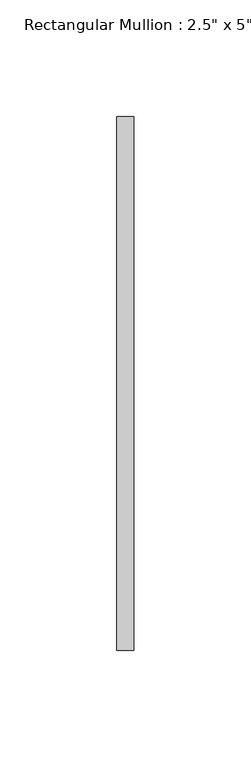
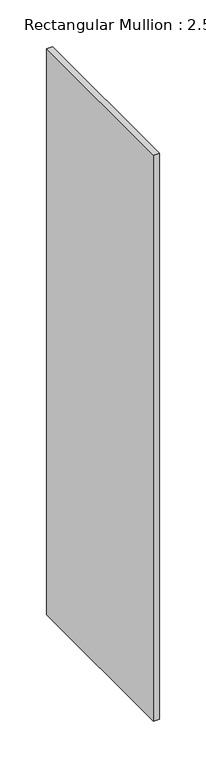
"""IFC4 building model written with IfcOpenShell, lengths in millimetres: member geometry."""

from ifc_helpers import new_model, si_unit, frame, origin, place, context, project, spatial, polyline, outline, extrude, source, transform, mapped, element, save


def member_c9ff8968(model_context):
    return source(origin(), model_context, "Body", "SweptSolid", [
        extrude(outline(polyline([(3.6195, 114.3), (3.6195, -114.3), (-3.6195, -114.3), (-3.6195, 114.3), (3.6195, 114.3)])), frame((0.0, 0.0, -738.4415), z_axis=(0.0, 0.0, 1.0), x_axis=(1.0, 0.0, 0.0)), (0.0, 0.0, 1.0), 738.4415),
    ])


if __name__ == "__main__":
    model = new_model("IFC4")
    model_context = context("Model", 3, world=origin())
    ifc_project = project(units=[si_unit("LENGTHUNIT", "METRE", prefix="MILLI")], contexts=[model_context])
    site = spatial("IfcSite", under=ifc_project)
    building = spatial("IfcBuilding", under=site)
    placement = place(None, origin())
    member_shape = member_c9ff8968(model_context)
    element("IfcMember", 1, ObjectType="Rectangular Mullion : 2.5\" x 5\" rectangular", at=placement, inside=building, context=model_context, shape_type="MappedRepresentation", body=[
        mapped(member_shape, transform((0.0, 0.0, 0.0), x_axis=(1.0, 0.0, 0.0), y_axis=(0.0, 1.0, 0.0), z_axis=(0.0, 0.0, 1.0))),
    ])
    save(model, "model.ifc")

# Revit data of these elements
# Type "Rectangular Mullion : 2.5\" x 5\" rectangular"
#   built-in parameter 1007304 = 0.75 (stored number, unit not read)
#   built-in parameter 1007301 = 0.011875 (stored number, unit not read)
#   built-in parameter 1007300 = 0.011875 (stored number, unit not read)
# Element 1 (IfcMember, "Rectangular Mullion : 2.5\" x 5\" rectangular")
#   Materials on its faces: "WINDOW GLASS MATERIAL"
# Materials
#   "WINDOW GLASS MATERIAL": class "Generic", colour RGB 120 120 120, transparency 0, Cost = 0
